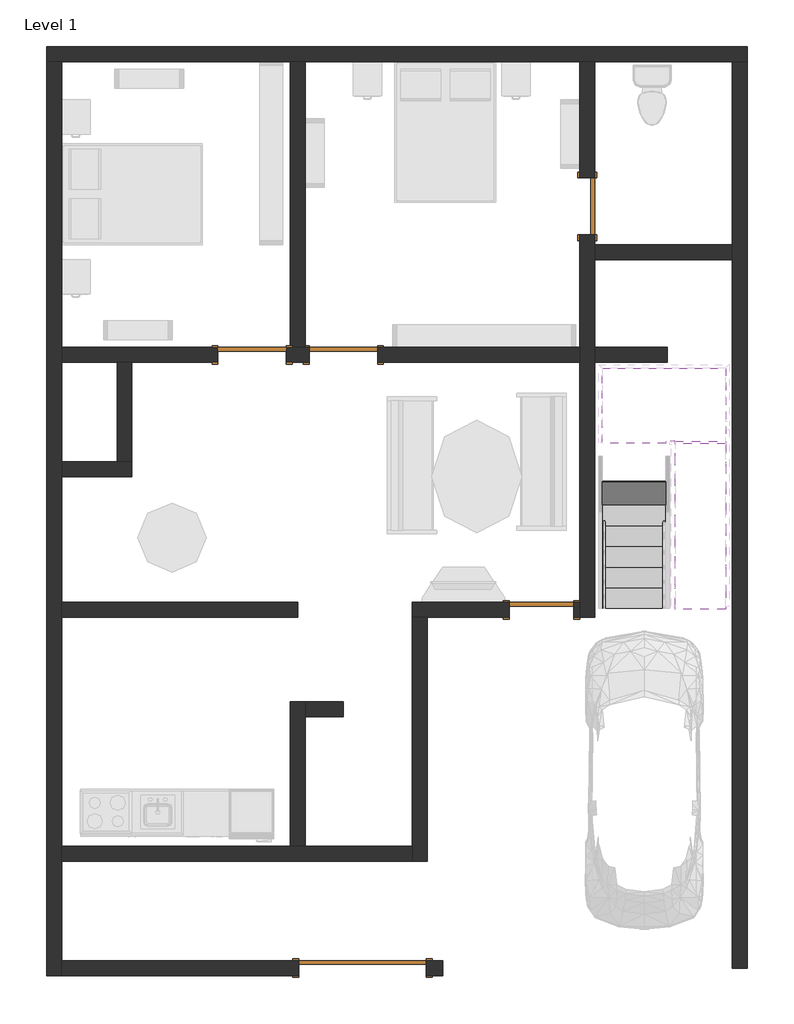
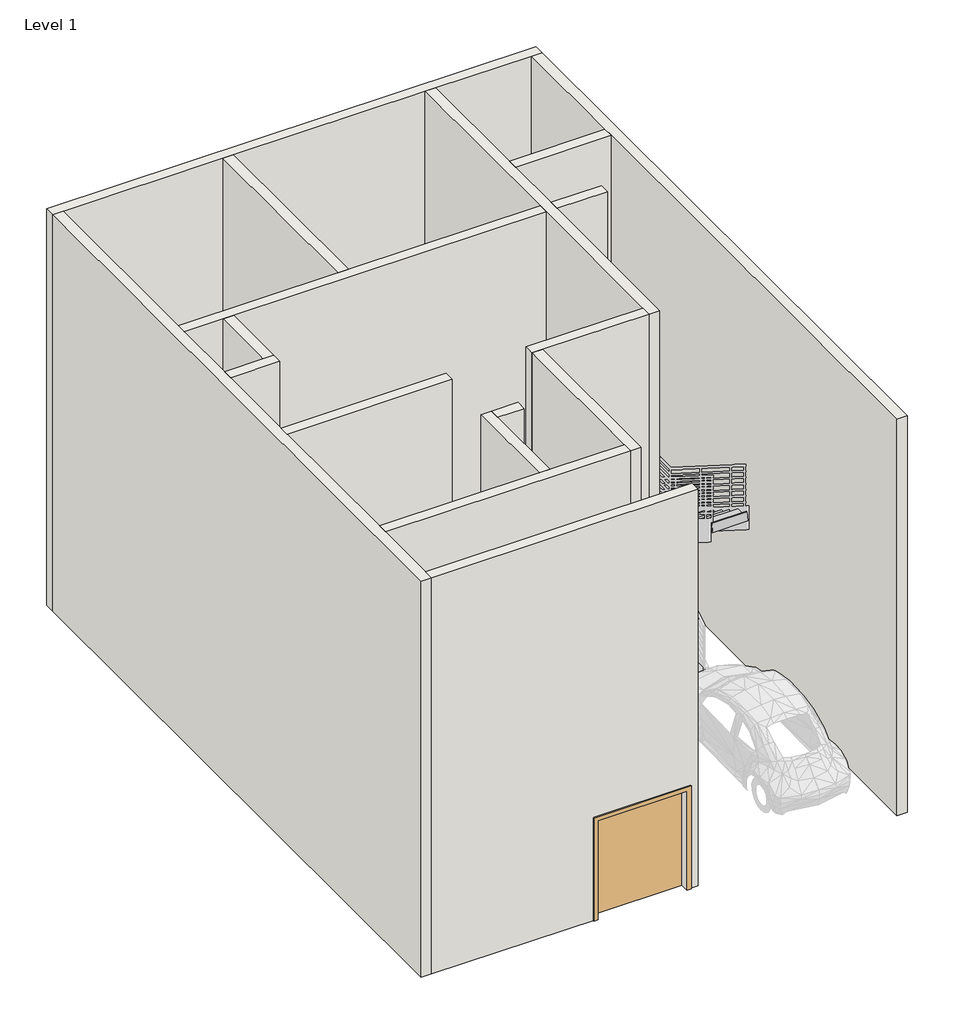
# One storey, part 1 of 4: 17 walls, 5 doors, 2 stair flights, 1 slab.
"""IFC4 building model written with IfcOpenShell, lengths in millimetres."""

from ifc_helpers import new_model, si_unit, frame, origin, origin_with_axes, place, context, project, spatial, polyline, outline, extrude, faceted_brep, transform, mapped, element, save
from components import m_door_double_flush_panel_double_acting_1700_x_2000mm_0a6d9c7f, m_single_flush_0762_x_2134mm_85379237, m_single_flush_0864_x_2134mm_5c09ce2c, m_single_flush_0915_x_2134mm_6a9e8738, m_single_flush_0915_x_2134mm_727434cd, non_monolithic_landing_8206a9fb, stair_flight_50mm_tread_25mm_nosing_13mm_riser_6f60bba3, stair_flight_50mm_tread_25mm_nosing_13mm_riser_fd2cf019

model = new_model("IFC4")

# Units and contexts
model_context = context("Model", 3, world=origin())
ifc_project = project(units=[si_unit("LENGTHUNIT", "METRE", prefix="MILLI")], contexts=[model_context])

# Site, building, storey
site = spatial("IfcSite", under=ifc_project)
building = spatial("IfcBuilding", under=site)
storey = spatial("IfcBuildingStorey", under=building, Name="Level 1", Elevation=0.0)

# Doors
placement = place(None, origin())
m_door_double_flush_panel_double_acting_1700_x_2000mm_shape = m_door_double_flush_panel_double_acting_1700_x_2000mm_0a6d9c7f(model_context)
element("IfcDoor", 1, ObjectType="M_Door-Double-Flush_Panel-Double-Acting : 1700 x 2000mm", at=placement, inside=storey, context=model_context, shape_type="MappedRepresentation", body=[
    mapped(m_door_double_flush_panel_double_acting_1700_x_2000mm_shape, transform((-3566.8389075, 322.0805518, 0.0), x_axis=(1.0, 0.0, 0.0), y_axis=(0.0, 1.0, 0.0), z_axis=(0.0, 0.0, 1.0))),
])
m_single_flush_0762_x_2134mm_shape = m_single_flush_0762_x_2134mm_85379237(model_context)
element("IfcDoor", 2, ObjectType="M_Single-Flush : 0762 x 2134mm", at=placement, inside=storey, context=model_context, shape_type="MappedRepresentation", body=[
    mapped(m_single_flush_0762_x_2134mm_shape, transform((-569.6389075, 10482.0805518, 0.0), x_axis=(0.0, -1.0, 0.0), y_axis=(1.0, 0.0, 0.0), z_axis=(0.0, 0.0, 1.0))),
])
m_single_flush_0864_x_2134mm_shape = m_single_flush_0864_x_2134mm_5c09ce2c(model_context)
element("IfcDoor", 3, ObjectType="M_Single-Flush : 0864 x 2134mm", at=placement, inside=storey, context=model_context, shape_type="MappedRepresentation", body=[
    mapped(m_single_flush_0864_x_2134mm_shape, transform((-1179.2389075, 5098.8805518, 0.0), x_axis=(1.0, 0.0, 0.0), y_axis=(0.0, 1.0, 0.0), z_axis=(0.0, 0.0, 1.0))),
])
m_single_flush_0915_x_2134mm_shape = m_single_flush_0915_x_2134mm_6a9e8738(model_context)
element("IfcDoor", 4, ObjectType="M_Single-Flush : 0915 x 2134mm", at=placement, inside=storey, context=model_context, shape_type="MappedRepresentation", body=[
    mapped(m_single_flush_0915_x_2134mm_shape, transform((-5040.0389075, 8500.8805518, 0.0), x_axis=(1.0, 0.0, 0.0), y_axis=(0.0, 1.0, 0.0), z_axis=(0.0, 0.0, 1.0))),
])
m_single_flush_0915_x_2134mm_2_shape = m_single_flush_0915_x_2134mm_727434cd(model_context)
element("IfcDoor", 5, ObjectType="M_Single-Flush : 0915 x 2134mm", at=placement, inside=storey, context=model_context, shape_type="MappedRepresentation", body=[
    mapped(m_single_flush_0915_x_2134mm_2_shape, transform((-3820.8389075, 8500.8805518, 0.0), x_axis=(-1.0, 0.0, 0.0), y_axis=(0.0, -1.0, 0.0), z_axis=(0.0, 0.0, 1.0))),
])

# Slab
non_monolithic_landing_shape = non_monolithic_landing_8206a9fb(model_context)
element("IfcSlab", 6, ObjectType="Non-Monolithic Landing", at=placement, inside=storey, context=model_context, shape_type="MappedRepresentation", body=[
    mapped(non_monolithic_landing_shape, transform((0.0, 0.0, 0.0), x_axis=(1.0, 0.0, 0.0), y_axis=(0.0, 1.0, 0.0), z_axis=(0.0, 0.0, 1.0))),
])

# Stair flights
stair_flight_50mm_tread_25mm_nosing_13mm_riser_shape = stair_flight_50mm_tread_25mm_nosing_13mm_riser_6f60bba3(model_context)
element("IfcStairFlight", 7, ObjectType="50mm Tread 25mm Nosing 13mm Riser", at=placement, inside=storey, context=model_context, shape_type="MappedRepresentation", body=[
    mapped(stair_flight_50mm_tread_25mm_nosing_13mm_riser_shape, transform((0.0, 0.0, 0.0), x_axis=(1.0, 0.0, 0.0), y_axis=(0.0, 1.0, 0.0), z_axis=(0.0, 0.0, 1.0))),
])
stair_flight_50mm_tread_25mm_nosing_13mm_riser_2_shape = stair_flight_50mm_tread_25mm_nosing_13mm_riser_fd2cf019(model_context)
element("IfcStairFlight", 8, ObjectType="50mm Tread 25mm Nosing 13mm Riser", at=placement, inside=storey, context=model_context, shape_type="MappedRepresentation", body=[
    mapped(stair_flight_50mm_tread_25mm_nosing_13mm_riser_2_shape, transform((0.0, 0.0, 0.0), x_axis=(1.0, 0.0, 0.0), y_axis=(0.0, 1.0, 0.0), z_axis=(0.0, 0.0, 1.0))),
])

# Walls
element("IfcWall", 9, ObjectType="Generic - 200mm", at=placement, inside=storey, context=model_context, shape_type="Brep", body=[
    faceted_brep([(-7781.6389075, 12414.0805518, 0.0), (-7581.6389075, 12414.0805518, 0.0), (-4530.4389075, 12414.0805518, 0.0), (-4330.4389075, 12414.0805518, 0.0), (-669.6389075, 12414.0805518, 0.0), (-469.6389075, 12414.0805518, 0.0), (1362.3610925, 12414.0805518, 0.0), (1562.3610925, 12414.0805518, 0.0), (1562.3610925, 12414.0805518, 8000.0), (1362.3610925, 12414.0805518, 8000.0), (-469.6389075, 12414.0805518, 8000.0), (-669.6389075, 12414.0805518, 8000.0), (-4330.4389075, 12414.0805518, 8000.0), (-4530.4389075, 12414.0805518, 8000.0), (-7581.6389075, 12414.0805518, 8000.0), (-7781.6389075, 12414.0805518, 8000.0), (-7781.6389075, 12614.0805518, 0.0), (-7781.6389075, 12614.0805518, 8000.0), (1562.3610925, 12614.0805518, 8000.0), (1562.3610925, 12614.0805518, 0.0)], [[[0, 1, 2, 3, 4, 5, 6, 7, 8, 9, 10, 11, 12, 13, 14, 15]], [[16, 17, 18, 19]], [[7, 6, 5, 4, 3, 2, 1, 0, 16, 19]], [[15, 14, 13, 12, 11, 10, 9, 8, 18, 17]], [[8, 7, 19, 18]], [[0, 15, 17, 16]]]),
])
element("IfcWall", 10, ObjectType="Generic - 200mm", at=placement, inside=storey, context=model_context, shape_type="Brep", body=[
    faceted_brep([(1362.3610925, 12414.0805518, 0.0), (1362.3610925, 9972.4805518, 0.0), (1362.3610925, 9772.4805518, 0.0), (1362.3610925, 322.0805518, 0.0), (1362.3610925, 322.0805518, 8000.0), (1362.3610925, 9772.4805518, 8000.0), (1362.3610925, 9972.4805518, 8000.0), (1362.3610925, 12414.0805518, 8000.0), (1562.3610925, 12414.0805518, 0.0), (1562.3610925, 12414.0805518, 8000.0), (1562.3610925, 322.0805518, 8000.0), (1562.3610925, 322.0805518, 0.0)], [[[0, 1, 2, 3, 4, 5, 6, 7]], [[8, 9, 10, 11]], [[3, 2, 1, 0, 8, 11]], [[4, 3, 11, 10]], [[7, 6, 5, 4, 10, 9]], [[0, 7, 9, 8]]]),
])
element("IfcWall", 11, ObjectType="Generic - 200mm", at=placement, inside=storey, context=model_context, shape_type="Brep", body=[
    faceted_brep([(-7581.6389075, 222.0805518, 0.0), (-7581.6389075, 422.0805518, 0.0), (-7581.6389075, 1746.0805518, 0.0), (-7581.6389075, 1946.0805518, 0.0), (-7581.6389075, 4998.8805518, 0.0), (-7581.6389075, 5198.8805518, 0.0), (-7581.6389075, 6876.8805518, 0.0), (-7581.6389075, 7076.8805518, 0.0), (-7581.6389075, 8400.8805518, 0.0), (-7581.6389075, 8600.8805518, 0.0), (-7581.6389075, 12414.0805518, 0.0), (-7581.6389075, 12414.0805518, 8000.0), (-7581.6389075, 8600.8805518, 8000.0), (-7581.6389075, 8400.8805518, 8000.0), (-7581.6389075, 7076.8805518, 8000.0), (-7581.6389075, 6876.8805518, 8000.0), (-7581.6389075, 5198.8805518, 8000.0), (-7581.6389075, 4998.8805518, 8000.0), (-7581.6389075, 1946.0805518, 8000.0), (-7581.6389075, 1746.0805518, 8000.0), (-7581.6389075, 422.0805518, 8000.0), (-7581.6389075, 222.0805518, 8000.0), (-7781.6389075, 222.0805518, 0.0), (-7781.6389075, 222.0805518, 8000.0), (-7781.6389075, 12414.0805518, 8000.0), (-7781.6389075, 12414.0805518, 0.0)], [[[0, 1, 2, 3, 4, 5, 6, 7, 8, 9, 10, 11, 12, 13, 14, 15, 16, 17, 18, 19, 20, 21]], [[22, 23, 24, 25]], [[10, 9, 8, 7, 6, 5, 4, 3, 2, 1, 0, 22, 25]], [[21, 20, 19, 18, 17, 16, 15, 14, 13, 12, 11, 24, 23]], [[11, 10, 25, 24]], [[0, 21, 23, 22]]]),
])
element("IfcWall", 12, ObjectType="Generic - 200mm", at=placement, inside=storey, context=model_context, shape_type="Brep", body=[
    faceted_brep([(-4582.5389075, 8400.8805518, 0.0), (-4278.3389075, 8400.8805518, 0.0), (-4278.3389075, 8400.8805518, 2134.0), (-3363.3389075, 8400.8805518, 2134.0), (-3363.3389075, 8400.8805518, 0.0), (-669.6389075, 8400.8805518, 0.0), (-669.6389075, 8400.8805518, 8000.0), (-6641.8389075, 8400.8805518, 8000.0), (-6841.8389075, 8400.8805518, 8000.0), (-7581.6389075, 8400.8805518, 8000.0), (-7581.6389075, 8400.8805518, 0.0), (-6841.8389075, 8400.8805518, 0.0), (-6641.8389075, 8400.8805518, 0.0), (-5497.5389075, 8400.8805518, 0.0), (-5497.5389075, 8400.8805518, 2134.0), (-4582.5389075, 8400.8805518, 2134.0), (-4278.3389075, 8600.8805518, 2134.0), (-4278.3389075, 8600.8805518, 0.0), (-4330.4389075, 8600.8805518, 0.0), (-4530.4389075, 8600.8805518, 0.0), (-4582.5389075, 8600.8805518, 0.0), (-4582.5389075, 8600.8805518, 2134.0), (-5497.5389075, 8600.8805518, 2134.0), (-5497.5389075, 8600.8805518, 0.0), (-7581.6389075, 8600.8805518, 0.0), (-7581.6389075, 8600.8805518, 8000.0), (-4530.4389075, 8600.8805518, 8000.0), (-4330.4389075, 8600.8805518, 8000.0), (-669.6389075, 8600.8805518, 8000.0), (-669.6389075, 8600.8805518, 0.0), (-3363.3389075, 8600.8805518, 0.0), (-3363.3389075, 8600.8805518, 2134.0)], [[[0, 1, 2, 3, 4, 5, 6, 7, 8, 9, 10, 11, 12, 13, 14, 15]], [[16, 17, 18, 19, 20, 21, 22, 23, 24, 25, 26, 27, 28, 29, 30, 31]], [[30, 29, 5, 4]], [[20, 19, 18, 17, 1, 0]], [[13, 12, 11, 10, 24, 23]], [[9, 8, 7, 6, 28, 27, 26, 25]], [[10, 9, 25, 24]], [[6, 5, 29, 28]], [[21, 20, 0, 15]], [[22, 21, 15, 14]], [[23, 22, 14, 13]], [[2, 1, 17, 16]], [[3, 2, 16, 31]], [[4, 3, 31, 30]]]),
])
element("IfcWall", 13, ObjectType="Generic - 200mm", at=placement, inside=storey, context=model_context, shape_type="SweptSolid", body=[
    extrude(outline(polyline([(-4330.4389075, 12414.0805518), (-4330.4389075, 8600.8805518), (-4530.4389075, 8600.8805518), (-4530.4389075, 12414.0805518), (-4330.4389075, 12414.0805518)])), origin_with_axes(), (0.0, 0.0, 1.0), 8000.0),
])
element("IfcWall", 14, ObjectType="Generic - 200mm", at=placement, inside=storey, context=model_context, shape_type="Brep", body=[
    faceted_brep([(-469.6389075, 4998.8805518, 0.0), (-469.6389075, 8400.8805518, 0.0), (-469.6389075, 8600.8805518, 0.0), (-469.6389075, 9772.4805518, 0.0), (-469.6389075, 9972.4805518, 0.0), (-469.6389075, 10101.0805518, 0.0), (-469.6389075, 10101.0805518, 2134.0), (-469.6389075, 10863.0805518, 2134.0), (-469.6389075, 10863.0805518, 0.0), (-469.6389075, 12414.0805518, 0.0), (-469.6389075, 12414.0805518, 8000.0), (-469.6389075, 9972.4805518, 8000.0), (-469.6389075, 9772.4805518, 8000.0), (-469.6389075, 8600.8805518, 8000.0), (-469.6389075, 8400.8805518, 8000.0), (-469.6389075, 4998.8805518, 8000.0), (-669.6389075, 10101.0805518, 2134.0), (-669.6389075, 10101.0805518, 0.0), (-669.6389075, 8600.8805518, 0.0), (-669.6389075, 8400.8805518, 0.0), (-669.6389075, 5198.8805518, 0.0), (-669.6389075, 4998.8805518, 0.0), (-669.6389075, 4998.8805518, 8000.0), (-669.6389075, 5198.8805518, 8000.0), (-669.6389075, 8400.8805518, 8000.0), (-669.6389075, 8600.8805518, 8000.0), (-669.6389075, 12414.0805518, 8000.0), (-669.6389075, 12414.0805518, 0.0), (-669.6389075, 10863.0805518, 0.0), (-669.6389075, 10863.0805518, 2134.0)], [[[0, 1, 2, 3, 4, 5, 6, 7, 8, 9, 10, 11, 12, 13, 14, 15]], [[16, 17, 18, 19, 20, 21, 22, 23, 24, 25, 26, 27, 28, 29]], [[28, 27, 9, 8]], [[21, 20, 19, 18, 17, 5, 4, 3, 2, 1, 0]], [[15, 14, 13, 12, 11, 10, 26, 25, 24, 23, 22]], [[10, 9, 27, 26]], [[6, 5, 17, 16]], [[7, 6, 16, 29]], [[8, 7, 29, 28]], [[0, 15, 22, 21]]]),
])
element("IfcWall", 15, ObjectType="Generic - 200mm", at=placement, inside=storey, context=model_context, shape_type="SweptSolid", body=[
    extrude(outline(polyline([(1362.3610925, 9772.4805518), (-469.6389075, 9772.4805518), (-469.6389075, 9972.4805518), (1362.3610925, 9972.4805518), (1362.3610925, 9772.4805518)])), origin_with_axes(), (0.0, 0.0, 1.0), 8000.0),
])
element("IfcWall", 16, ObjectType="Generic - 200mm", at=placement, inside=storey, context=model_context, shape_type="Brep", body=[
    faceted_brep([(-7581.6389075, 6876.8805518, 0.0), (-6641.8389075, 6876.8805518, 0.0), (-6641.8389075, 6876.8805518, 8000.0), (-7581.6389075, 6876.8805518, 8000.0), (-7581.6389075, 7076.8805518, 0.0), (-7581.6389075, 7076.8805518, 8000.0), (-6841.8389075, 7076.8805518, 8000.0), (-6641.8389075, 7076.8805518, 8000.0), (-6641.8389075, 7076.8805518, 0.0), (-6841.8389075, 7076.8805518, 0.0)], [[[0, 1, 2, 3]], [[4, 5, 6, 7, 8, 9]], [[1, 0, 4, 9, 8]], [[3, 2, 7, 6, 5]], [[0, 3, 5, 4]], [[2, 1, 8, 7]]]),
])
element("IfcWall", 17, ObjectType="Generic - 200mm", at=placement, inside=storey, context=model_context, shape_type="SweptSolid", body=[
    extrude(outline(polyline([(-6641.8389075, 8400.8805518), (-6641.8389075, 7076.8805518), (-6841.8389075, 7076.8805518), (-6841.8389075, 8400.8805518), (-6641.8389075, 8400.8805518)])), origin_with_axes(), (0.0, 0.0, 1.0), 8000.0),
])
element("IfcWall", 18, ObjectType="Generic - 200mm", at=placement, inside=storey, context=model_context, shape_type="SweptSolid", body=[
    extrude(outline(polyline([(-4430.4389075, 4998.8805518), (-7581.6389075, 4998.8805518), (-7581.6389075, 5198.8805518), (-4430.4389075, 5198.8805518), (-4430.4389075, 4998.8805518)])), origin_with_axes(), (0.0, 0.0, 1.0), 8000.0),
])
element("IfcWall", 19, ObjectType="Generic - 200mm", at=placement, inside=storey, context=model_context, shape_type="Brep", body=[
    faceted_brep([(-669.6389075, 5198.8805518, 0.0), (-747.2389075, 5198.8805518, 0.0), (-747.2389075, 5198.8805518, 2134.0), (-1611.2389075, 5198.8805518, 2134.0), (-1611.2389075, 5198.8805518, 0.0), (-2904.8389075, 5198.8805518, 0.0), (-2904.8389075, 5198.8805518, 8000.0), (-669.6389075, 5198.8805518, 8000.0), (-747.2389075, 4998.8805518, 2134.0), (-747.2389075, 4998.8805518, 0.0), (-669.6389075, 4998.8805518, 0.0), (-669.6389075, 4998.8805518, 8000.0), (-2704.8389075, 4998.8805518, 8000.0), (-2904.8389075, 4998.8805518, 8000.0), (-2904.8389075, 4998.8805518, 0.0), (-2704.8389075, 4998.8805518, 0.0), (-1611.2389075, 4998.8805518, 0.0), (-1611.2389075, 4998.8805518, 2134.0)], [[[0, 1, 2, 3, 4, 5, 6, 7]], [[8, 9, 10, 11, 12, 13, 14, 15, 16, 17]], [[10, 9, 1, 0]], [[16, 15, 14, 5, 4]], [[7, 6, 13, 12, 11]], [[0, 7, 11, 10]], [[2, 1, 9, 8]], [[3, 2, 8, 17]], [[4, 3, 17, 16]], [[6, 5, 14, 13]]]),
])
element("IfcWall", 20, ObjectType="Generic - 200mm", at=placement, inside=storey, context=model_context, shape_type="SweptSolid", body=[
    extrude(outline(polyline([(497.1610925, 8400.8805518), (-469.6389075, 8400.8805518), (-469.6389075, 8600.8805518), (497.1610925, 8600.8805518), (497.1610925, 8400.8805518)])), origin_with_axes(), (0.0, 0.0, 1.0), 8000.0),
])
element("IfcWall", 21, ObjectType="Generic - 200mm", at=placement, inside=storey, context=model_context, shape_type="Brep", body=[
    faceted_brep([(-7581.6389075, 1746.0805518, 0.0), (-2904.8389075, 1746.0805518, 0.0), (-2904.8389075, 1746.0805518, 8000.0), (-7581.6389075, 1746.0805518, 8000.0), (-7581.6389075, 1946.0805518, 0.0), (-7581.6389075, 1946.0805518, 8000.0), (-4530.4389075, 1946.0805518, 8000.0), (-4330.4389075, 1946.0805518, 8000.0), (-2904.8389075, 1946.0805518, 8000.0), (-2904.8389075, 1946.0805518, 0.0), (-4330.4389075, 1946.0805518, 0.0), (-4530.4389075, 1946.0805518, 0.0)], [[[0, 1, 2, 3]], [[4, 5, 6, 7, 8, 9, 10, 11]], [[1, 0, 4, 11, 10, 9]], [[3, 2, 8, 7, 6, 5]], [[0, 3, 5, 4]], [[2, 1, 9, 8]]]),
])
element("IfcWall", 22, ObjectType="Generic - 200mm", at=placement, inside=storey, context=model_context, shape_type="Brep", body=[
    faceted_brep([(-4330.4389075, 1946.0805518, 0.0), (-4330.4389075, 3676.4805518, 0.0), (-4330.4389075, 3876.4805518, 0.0), (-4330.4389075, 3876.4805518, 8000.0), (-4330.4389075, 3676.4805518, 8000.0), (-4330.4389075, 1946.0805518, 8000.0), (-4530.4389075, 1946.0805518, 0.0), (-4530.4389075, 1946.0805518, 8000.0), (-4530.4389075, 3876.4805518, 8000.0), (-4530.4389075, 3876.4805518, 0.0)], [[[0, 1, 2, 3, 4, 5]], [[6, 7, 8, 9]], [[2, 1, 0, 6, 9]], [[5, 4, 3, 8, 7]], [[0, 5, 7, 6]], [[3, 2, 9, 8]]]),
])
element("IfcWall", 23, ObjectType="Generic - 200mm", at=placement, inside=storey, context=model_context, shape_type="SweptSolid", body=[
    extrude(outline(polyline([(-3820.8389075, 3676.4805518), (-4330.4389075, 3676.4805518), (-4330.4389075, 3876.4805518), (-3820.8389075, 3876.4805518), (-3820.8389075, 3676.4805518)])), origin_with_axes(), (0.0, 0.0, 1.0), 8000.0),
])
element("IfcWall", 24, ObjectType="Generic - 200mm", at=placement, inside=storey, context=model_context, shape_type="Brep", body=[
    faceted_brep([(-2904.8389075, 4998.8805518, 0.0), (-2904.8389075, 1946.0805518, 0.0), (-2904.8389075, 1746.0805518, 0.0), (-2904.8389075, 1746.0805518, 8000.0), (-2904.8389075, 1946.0805518, 8000.0), (-2904.8389075, 4998.8805518, 8000.0), (-2704.8389075, 4998.8805518, 0.0), (-2704.8389075, 4998.8805518, 8000.0), (-2704.8389075, 1746.0805518, 8000.0), (-2704.8389075, 1746.0805518, 0.0)], [[[0, 1, 2, 3, 4, 5]], [[6, 7, 8, 9]], [[2, 1, 0, 6, 9]], [[5, 4, 3, 8, 7]], [[0, 5, 7, 6]], [[3, 2, 9, 8]]]),
])
element("IfcWall", 25, ObjectType="Generic - 200mm", at=placement, inside=storey, context=model_context, shape_type="SweptSolid", body=[
    extrude(outline(polyline([(0.0, -2500.0389075), (8000.0, -2500.0389075), (8000.0, -7581.6389075), (0.0, -7581.6389075), (0.0, -4416.8389075), (2000.0, -4416.8389075), (2000.0, -2716.8389075), (0.0, -2716.8389075), (0.0, -2500.0389075)])), frame((0.0, 222.0805518, 0.0), z_axis=(0.0, 1.0, 0.0), x_axis=(0.0, 0.0, 1.0)), (0.0, 0.0, 1.0), 200.0),
])

save(model, "model.ifc")

# Revit data of these elements
# Type "M_Door-Double-Flush_Panel-Double-Acting : 1700 x 2000mm"
#   Type Mark = "22"
#   Construction Type Id = "DOOR"
#   Assembly Code = "C1020"
#   Analytic Construction = "Wooden"
#   W = 850 mm
#   Thickness = 50 mm
#   Thermal Resistance (R) = 0.455703 (m²·K)/W
#   Swing Angle [instance default] = 90.00°
#   Heat Transfer Coefficient (U) = 2.19465 W/(m²·K)
#   Height = 2000 mm
#   Trim Projection Ext. = 25 mm
#   Trim Projection Int. = 25 mm
#   Trim Width Ext. = 80 mm
#   Trim Width Int. = 80 mm
#   Width = 1700 mm
#   Define Thermal Properties by = 1
#   Panel Material = Wood - Birch - Solid Stained Light Low Gloss
#   Trim Material = Paint - Sienna
#   Visual Light Transmittance = 0
#   Solar Heat Gain Coefficient = 0
#   Function = (empty or 0)
#   Wall Closure = (empty or 0)
# Type "M_Single-Flush : 0762 x 2134mm"
#   Type Mark = "18"
#   Thickness = 51 mm
#   Height = 2134 mm
#   Trim Projection Ext = 25 mm
#   Trim Projection Int = 25 mm
#   Trim Width = 76 mm
#   Width = 762 mm
#   Door Material = Door - Panel
#   Frame Material = Door - Frame
#   Function = (empty or 0)
#   Wall Closure = (empty or 0)
# Type "M_Single-Flush : 0864 x 2134mm"
#   Type Mark = "16"
#   Thickness = 51 mm
#   Height = 2134 mm
#   Trim Projection Ext = 25 mm
#   Trim Projection Int = 25 mm
#   Trim Width = 76 mm
#   Width = 864 mm
#   Door Material = Door - Panel
#   Frame Material = Door - Frame
#   Function = (empty or 0)
#   Wall Closure = (empty or 0)
# Type "M_Single-Flush : 0915 x 2134mm"
#   Type Mark = "15"
#   Thickness = 51 mm
#   Height = 2134 mm
#   Trim Projection Ext = 25 mm
#   Trim Projection Int = 25 mm
#   Trim Width = 76 mm
#   Width = 915 mm
#   Door Material = Door - Panel
#   Frame Material = Door - Frame
#   Function = (empty or 0)
#   Wall Closure = (empty or 0)
# Type "Generic - 200mm"
#   Layers, outside or top first: 200 mm no material (function 1)
# Element 1 (IfcDoor, "M_Door-Double-Flush_Panel-Double-Acting : 1700 x 2000mm")
#   Swing Angle = 90.00°
#   Phase Created = New Construction
#   Materials on its faces: "Paint - Sienna", "Wood - Birch - Solid Stained Light Low Gloss"
# Element 2 (IfcDoor, "M_Single-Flush : 0762 x 2134mm")
#   Phase Created = New Construction
#   Materials on its faces: "Door - Frame", "Door - Panel"
# Element 3 (IfcDoor, "M_Single-Flush : 0864 x 2134mm")
#   Phase Created = New Construction
#   Materials on its faces: "Door - Frame", "Door - Panel"
# Elements 4, 5 (IfcDoor, "M_Single-Flush : 0915 x 2134mm")
#   Phase Created = New Construction
#   Materials on its faces: "Door - Frame", "Door - Panel"
# Element 6 (IfcSlab, "Non-Monolithic Landing")
#   Phase Created = New Construction
# Elements 7, 8 (IfcStairFlight, "50mm Tread 25mm Nosing 13mm Riser")
#   Phase Created = New Construction
# Elements 9, 10, 11, 12, 13, 14, 15, 16, 17, 18, 19, 20, 21, 22, 23, 24, 25 (IfcWall, "Generic - 200mm")
#   Top Offset = 0 mm
#   Base Offset = 0 mm
#   Unconnected Height = 8000 mm
#   wall height = 8000 mm
#   Phase Created = New Construction
#   Base Constraint = Level 1
#   Materials on its faces: "Default Wall"
# Materials
#   "Wood - Birch - Solid Stained Light Low Gloss": class "Wood", colour RGB 210 159 95, transparency 0, Cost = 0
#   "Paint - Sienna": colour RGB 118 70 51, transparency 0, Cost = 0
#   "Door - Panel": class "Wood", colour RGB 114 82 51, transparency 0
#   "Door - Frame": colour RGB 153 76 43, transparency 0
#   "Default Wall": colour RGB 80 80 80, transparency 0
